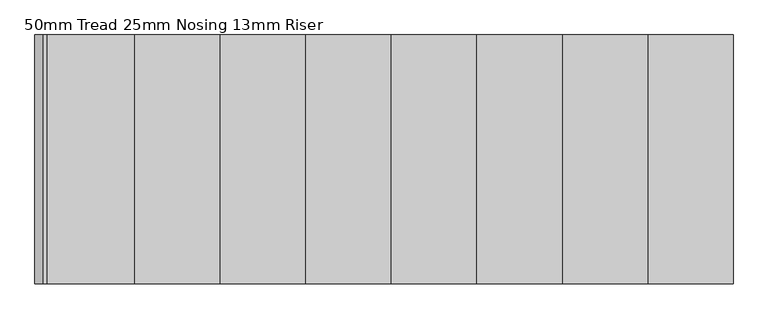
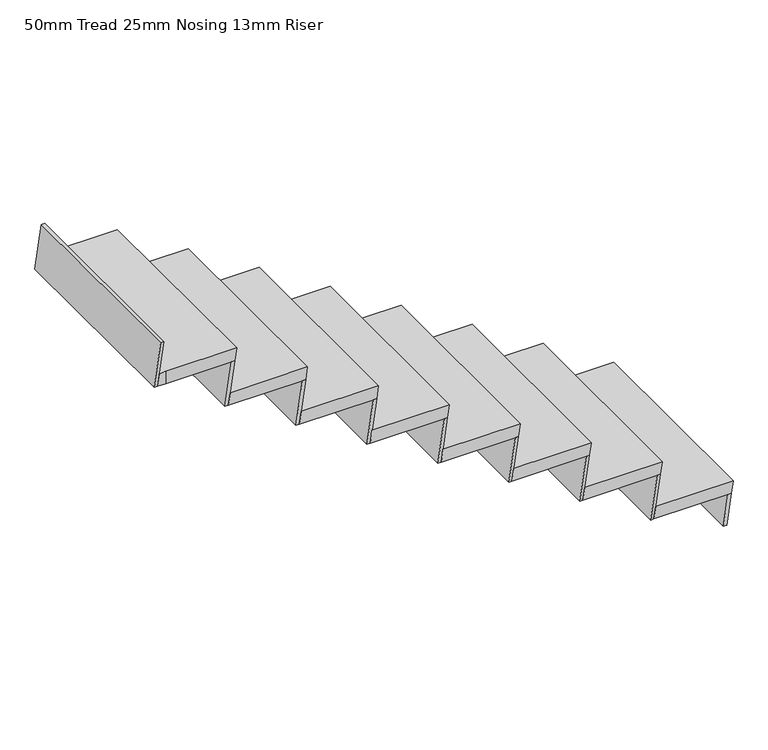
"""IFC4 building model written with IfcOpenShell, lengths in millimetres: stair flight geometry, 50mm Tread 25mm Nosing 13mm Riser."""

from ifc_helpers import new_model, si_unit, origin, place, context, project, spatial, faceted_brep, source, transform, mapped, element, save


def stair_flight_50mm_tread_25mm_nosing_13mm_riser_b8c52427(model_context):
    return source(origin(), model_context, "Body", "Brep", [
        faceted_brep([(-7453.6870075, 2212.3123547, 173.9130435), (-7460.8745075, 2212.3123547, 123.9130435), (-7460.8745075, 1412.2865734, 123.9130435), (-7453.6870075, 1412.2865734, 173.9130435), (-7153.6870075, 1412.2865734, 173.9130435), (-7153.6870075, 2212.3123547, 173.9130435), (-7160.8745075, 2212.3123547, 123.9130435), (-7160.8745075, 1412.2865734, 123.9130435)], [[[0, 1, 2, 3]], [[3, 4, 5, 0]], [[2, 1, 6, 7]], [[4, 3, 2, 7]], [[0, 5, 6, 1]], [[5, 4, 7, 6]]]),
        faceted_brep([(-7160.8745075, 2212.3123547, 123.9130435), (-7178.6870075, 2212.3123547, 0.0), (-7191.3154975, 2212.3123547, 0.0), (-7173.5029975, 2212.3123547, 123.9130435), (-7160.8745075, 1412.2865734, 123.9130435), (-7173.5029975, 1412.2865734, 123.9130435), (-7191.3154975, 1412.2865734, 0.0), (-7178.6870075, 1412.2865734, 0.0)], [[[0, 1, 2, 3]], [[4, 5, 6, 7]], [[1, 0, 4, 7]], [[2, 1, 7, 6]], [[3, 2, 6, 5]], [[0, 3, 5, 4]]]),
        faceted_brep([(-7435.8745075, 2212.3123547, 297.826087), (-7460.8745075, 2212.3123547, 123.9130435), (-7473.5029975, 2212.3123547, 123.9130435), (-7448.5029975, 2212.3123547, 297.826087), (-7435.8745075, 1412.2865734, 297.826087), (-7448.5029975, 1412.2865734, 297.826087), (-7473.5029975, 1412.2865734, 123.9130435), (-7460.8745075, 1412.2865734, 123.9130435)], [[[0, 1, 2, 3]], [[4, 5, 6, 7]], [[1, 0, 4, 7]], [[2, 1, 7, 6]], [[3, 2, 6, 5]], [[0, 3, 5, 4]]]),
        faceted_brep([(-7728.6870075, 1412.2865734, 347.826087), (-7428.6870075, 1412.2865734, 347.826087), (-7428.6870075, 2212.3123547, 347.826087), (-7728.6870075, 2212.3123547, 347.826087), (-7735.8745075, 1412.2865734, 297.826087), (-7735.8745075, 2212.3123547, 297.826087), (-7435.8745075, 2212.3123547, 297.826087), (-7435.8745075, 1412.2865734, 297.826087)], [[[0, 1, 2, 3]], [[4, 5, 6, 7]], [[1, 0, 4, 7]], [[3, 2, 6, 5]], [[3, 5, 4, 0]], [[2, 1, 7, 6]]]),
        faceted_brep([(-7710.8745075, 2212.3123547, 471.7391304), (-7735.8745075, 2212.3123547, 297.826087), (-7748.5029975, 2212.3123547, 297.826087), (-7723.5029975, 2212.3123547, 471.7391304), (-7710.8745075, 1412.2865734, 471.7391304), (-7723.5029975, 1412.2865734, 471.7391304), (-7748.5029975, 1412.2865734, 297.826087), (-7735.8745075, 1412.2865734, 297.826087)], [[[0, 1, 2, 3]], [[4, 5, 6, 7]], [[1, 0, 4, 7]], [[2, 1, 7, 6]], [[3, 2, 6, 5]], [[0, 3, 5, 4]]]),
        faceted_brep([(-8003.6870075, 1412.2865734, 521.7391304), (-7703.6870075, 1412.2865734, 521.7391304), (-7703.6870075, 2212.3123547, 521.7391304), (-8003.6870075, 2212.3123547, 521.7391304), (-8010.8745075, 1412.2865734, 471.7391304), (-8010.8745075, 2212.3123547, 471.7391304), (-7710.8745075, 2212.3123547, 471.7391304), (-7710.8745075, 1412.2865734, 471.7391304)], [[[0, 1, 2, 3]], [[4, 5, 6, 7]], [[1, 0, 4, 7]], [[3, 2, 6, 5]], [[3, 5, 4, 0]], [[2, 1, 7, 6]]]),
        faceted_brep([(-7985.8745075, 2212.3123547, 645.6521739), (-8010.8745075, 2212.3123547, 471.7391304), (-8023.5029975, 2212.3123547, 471.7391304), (-7998.5029975, 2212.3123547, 645.6521739), (-7985.8745075, 1412.2865734, 645.6521739), (-7998.5029975, 1412.2865734, 645.6521739), (-8023.5029975, 1412.2865734, 471.7391304), (-8010.8745075, 1412.2865734, 471.7391304)], [[[0, 1, 2, 3]], [[4, 5, 6, 7]], [[1, 0, 4, 7]], [[2, 1, 7, 6]], [[3, 2, 6, 5]], [[0, 3, 5, 4]]]),
        faceted_brep([(-8278.6870075, 1412.2865734, 695.6521739), (-7978.6870075, 1412.2865734, 695.6521739), (-7978.6870075, 2212.3123547, 695.6521739), (-8278.6870075, 2212.3123547, 695.6521739), (-8285.8745075, 1412.2865734, 645.6521739), (-8285.8745075, 2212.3123547, 645.6521739), (-7985.8745075, 2212.3123547, 645.6521739), (-7985.8745075, 1412.2865734, 645.6521739)], [[[0, 1, 2, 3]], [[4, 5, 6, 7]], [[1, 0, 4, 7]], [[3, 2, 6, 5]], [[3, 5, 4, 0]], [[2, 1, 7, 6]]]),
        faceted_brep([(-8260.8745075, 2212.3123547, 819.5652174), (-8285.8745075, 2212.3123547, 645.6521739), (-8298.5029975, 2212.3123547, 645.6521739), (-8273.5029975, 2212.3123547, 819.5652174), (-8260.8745075, 1412.2865734, 819.5652174), (-8273.5029975, 1412.2865734, 819.5652174), (-8298.5029975, 1412.2865734, 645.6521739), (-8285.8745075, 1412.2865734, 645.6521739)], [[[0, 1, 2, 3]], [[4, 5, 6, 7]], [[1, 0, 4, 7]], [[2, 1, 7, 6]], [[3, 2, 6, 5]], [[0, 3, 5, 4]]]),
        faceted_brep([(-8553.6870075, 1412.2865734, 869.5652174), (-8253.6870075, 1412.2865734, 869.5652174), (-8253.6870075, 2212.3123547, 869.5652174), (-8553.6870075, 2212.3123547, 869.5652174), (-8560.8745075, 1412.2865734, 819.5652174), (-8560.8745075, 2212.3123547, 819.5652174), (-8260.8745075, 2212.3123547, 819.5652174), (-8260.8745075, 1412.2865734, 819.5652174)], [[[0, 1, 2, 3]], [[4, 5, 6, 7]], [[1, 0, 4, 7]], [[3, 2, 6, 5]], [[3, 5, 4, 0]], [[2, 1, 7, 6]]]),
        faceted_brep([(-8535.8745075, 2212.3123547, 993.4782609), (-8560.8745075, 2212.3123547, 819.5652174), (-8573.5029975, 2212.3123547, 819.5652174), (-8548.5029975, 2212.3123547, 993.4782609), (-8535.8745075, 1412.2865734, 993.4782609), (-8548.5029975, 1412.2865734, 993.4782609), (-8573.5029975, 1412.2865734, 819.5652174), (-8560.8745075, 1412.2865734, 819.5652174)], [[[0, 1, 2, 3]], [[4, 5, 6, 7]], [[1, 0, 4, 7]], [[2, 1, 7, 6]], [[3, 2, 6, 5]], [[0, 3, 5, 4]]]),
        faceted_brep([(-8828.6870075, 1412.2865734, 1043.4782609), (-8528.6870075, 1412.2865734, 1043.4782609), (-8528.6870075, 2212.3123547, 1043.4782609), (-8828.6870075, 2212.3123547, 1043.4782609), (-8835.8745075, 1412.2865734, 993.4782609), (-8835.8745075, 2212.3123547, 993.4782609), (-8535.8745075, 2212.3123547, 993.4782609), (-8535.8745075, 1412.2865734, 993.4782609)], [[[0, 1, 2, 3]], [[4, 5, 6, 7]], [[1, 0, 4, 7]], [[3, 2, 6, 5]], [[3, 5, 4, 0]], [[2, 1, 7, 6]]]),
        faceted_brep([(-8810.8745075, 2212.3123547, 1167.3913043), (-8835.8745075, 2212.3123547, 993.4782609), (-8848.5029975, 2212.3123547, 993.4782609), (-8823.5029975, 2212.3123547, 1167.3913043), (-8810.8745075, 1412.2865734, 1167.3913043), (-8823.5029975, 1412.2865734, 1167.3913043), (-8848.5029975, 1412.2865734, 993.4782609), (-8835.8745075, 1412.2865734, 993.4782609)], [[[0, 1, 2, 3]], [[4, 5, 6, 7]], [[1, 0, 4, 7]], [[2, 1, 7, 6]], [[3, 2, 6, 5]], [[0, 3, 5, 4]]]),
        faceted_brep([(-9103.6870075, 1412.2865734, 1217.3913043), (-8803.6870075, 1412.2865734, 1217.3913043), (-8803.6870075, 2212.3123547, 1217.3913043), (-9103.6870075, 2212.3123547, 1217.3913043), (-9110.8745075, 1412.2865734, 1167.3913043), (-9110.8745075, 2212.3123547, 1167.3913043), (-8810.8745075, 2212.3123547, 1167.3913043), (-8810.8745075, 1412.2865734, 1167.3913043)], [[[0, 1, 2, 3]], [[4, 5, 6, 7]], [[1, 0, 4, 7]], [[3, 2, 6, 5]], [[3, 5, 4, 0]], [[2, 1, 7, 6]]]),
        faceted_brep([(-9360.8745075, 2212.3123547, 1515.2173913), (-9385.8745075, 2212.3123547, 1341.3043478), (-9398.5029975, 2212.3123547, 1341.3043478), (-9373.5029975, 2212.3123547, 1515.2173913), (-9360.8745075, 1412.2865734, 1515.2173913), (-9373.5029975, 1412.2865734, 1515.2173913), (-9398.5029975, 1412.2865734, 1341.3043478), (-9385.8745075, 1412.2865734, 1341.3043478)], [[[0, 1, 2, 3]], [[4, 5, 6, 7]], [[1, 0, 4, 7]], [[2, 1, 7, 6]], [[3, 2, 6, 5]], [[0, 3, 5, 4]]]),
        faceted_brep([(-9085.8745075, 2212.3123547, 1341.3043478), (-9110.8745075, 2212.3123547, 1167.3913043), (-9123.5029975, 2212.3123547, 1167.3913043), (-9098.5029975, 2212.3123547, 1341.3043478), (-9085.8745075, 1412.2865734, 1341.3043478), (-9098.5029975, 1412.2865734, 1341.3043478), (-9123.5029975, 1412.2865734, 1167.3913043), (-9110.8745075, 1412.2865734, 1167.3913043)], [[[0, 1, 2, 3]], [[4, 5, 6, 7]], [[1, 0, 4, 7]], [[2, 1, 7, 6]], [[3, 2, 6, 5]], [[0, 3, 5, 4]]]),
        faceted_brep([(-9378.6870075, 1412.2865734, 1391.3043478), (-9353.6870075, 1412.2865734, 1391.3043478), (-9078.6870075, 1412.2865734, 1391.3043478), (-9078.6870075, 2212.3123547, 1391.3043478), (-9378.6870075, 2212.3123547, 1391.3043478), (-9385.8745075, 1412.2865734, 1341.3043478), (-9385.8745075, 2212.3123547, 1341.3043478), (-9085.8745075, 2212.3123547, 1341.3043478), (-9085.8745075, 1412.2865734, 1341.3043478), (-9353.6870075, 1412.2865734, 1341.3043478)], [[[0, 1, 2, 3, 4]], [[5, 6, 7, 8, 9]], [[1, 0, 5, 9]], [[2, 1, 9, 8]], [[4, 3, 7, 6]], [[4, 6, 5, 0]], [[3, 2, 8, 7]]]),
    ])


if __name__ == "__main__":
    model = new_model("IFC4")
    model_context = context("Model", 3, world=origin())
    ifc_project = project(units=[si_unit("LENGTHUNIT", "METRE", prefix="MILLI")], contexts=[model_context])
    site = spatial("IfcSite", under=ifc_project)
    building = spatial("IfcBuilding", under=site)
    placement = place(None, origin())
    stair_flight_50mm_tread_25mm_nosing_13mm_riser_shape = stair_flight_50mm_tread_25mm_nosing_13mm_riser_b8c52427(model_context)
    element("IfcStairFlight", 1, ObjectType="50mm Tread 25mm Nosing 13mm Riser", at=placement, inside=building, context=model_context, shape_type="MappedRepresentation", body=[
        mapped(stair_flight_50mm_tread_25mm_nosing_13mm_riser_shape, transform((0.0, 0.0, 0.0), x_axis=(1.0, 0.0, 0.0), y_axis=(0.0, 1.0, 0.0), z_axis=(0.0, 0.0, 1.0))),
    ])
    save(model, "model.ifc")
